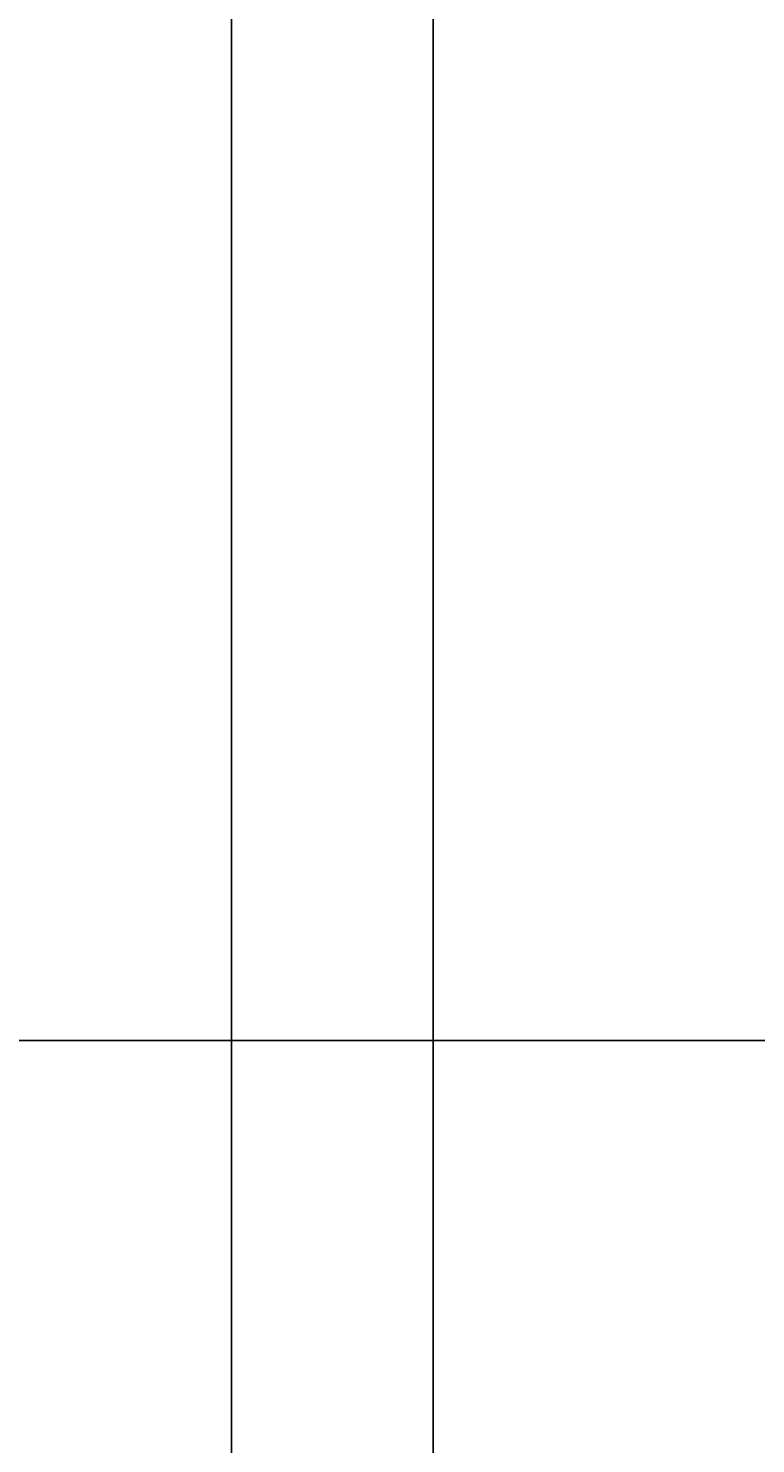
# Model space of a CAD drawing. Units: inches. Extents: x 37 to 706, y -568 to 110.
# Tile 13 of 24: x 494 to 526, y -468 to -405. Entities that reach past the tile are written whole.
import ezdxf

# ---------------------------------------------------------------- set-up
doc = ezdxf.new("R2010")
doc.units = ezdxf.units.IN
doc.header["$MEASUREMENT"] = 0
doc.layers.add('A-ANNO-DIMS', color=2, linetype='Continuous', lineweight=18)
doc.styles.get("Standard").update_dxf_attribs({"font": 'arial.ttf'})
doc.dimstyles.get("Standard").update_dxf_attribs({"dimtxt": 0.18, "dimasz": 0.18, "dimexe": 0.18, "dimexo": 0.0625, "dimgap": 0.09, "dimtad": 0, "dimtih": 1, "dimtoh": 1, "dimdec": 0, "dimzin": 0, "dimdsep": 46, "dimlunit": 3, "dimtxsty": 'Standard', "dimcen": 0.09, "dimadec": 0, "dimazin": 0, "dimtfac": 1, "dimtdec": 0, "dimtofl": 0, "dimtmove": 0, "dimatfit": 3, "dimfxl": 1, "dimtolj": 1, "dimtzin": 0, "dimarcsym": 0})

# ---------------------------------------------------------------- blocks, each defined once
blk = doc.blocks.new('*D45')
at = {"layer": 'A-ANNO-DIMS', "color": 0, "lineweight": -2, "transparency": 16777216}
for p, q in [((88.021, -449.708), (705.888, -449.708)), ((705.708, -449.888), (705.708, -481.527)), ((705.708, -513.528), (705.708, -481.89)), ((79.021, -513.708), (705.888, -513.708))]:
    blk.add_line(p, q, dxfattribs=at)
at = {"layer": 'A-ANNO-DIMS', "color": 0, "transparency": 16777216}
for points in [[(705.678, -449.888), (705.738, -449.888), (705.708, -449.708)], [(705.678, -513.528), (705.738, -513.528), (705.708, -513.708)]]:
    blk.add_solid(points, dxfattribs=at)
at = {"layer": 'Defpoints', "color": 0, "transparency": 16777216}
for p in [(87.958, -449.708), (705.708, -449.708), (78.958, -513.708)]:
    blk.add_point(p, dxfattribs=at)
at = {"layer": 'A-ANNO-DIMS', "color": 0, "transparency": 16777216, "insert": (705.708, -481.708), "char_height": 0.18, "attachment_point": 5}
blk.add_mtext('\\A1;5\'-4"', dxfattribs=at)
blk = doc.blocks.new('*D53')
at = {"layer": 'A-ANNO-DIMS', "color": 0, "lineweight": -2, "transparency": 16777216}
for p, q in [((511.958, -151.771), (511.958, -567.638)), ((537.958, -151.771), (537.958, -567.638)), ((512.138, -567.458), (524.628, -567.458)), ((537.778, -567.458), (525.289, -567.458))]:
    blk.add_line(p, q, dxfattribs=at)
at = {"layer": 'A-ANNO-DIMS', "color": 0, "transparency": 16777216}
for points in [[(512.138, -567.428), (512.138, -567.488), (511.958, -567.458)], [(537.778, -567.428), (537.778, -567.488), (537.958, -567.458)]]:
    blk.add_solid(points, dxfattribs=at)
at = {"layer": 'Defpoints', "color": 0, "transparency": 16777216}
for p in [(511.958, -151.708), (537.958, -151.708), (537.958, -567.458)]:
    blk.add_point(p, dxfattribs=at)
at = {"layer": 'A-ANNO-DIMS', "color": 0, "transparency": 16777216, "insert": (524.958, -567.458), "char_height": 0.18, "attachment_point": 5}
blk.add_mtext('\\A1;2\'-2"', dxfattribs=at)
blk = doc.blocks.new('*D63')
at = {"layer": 'A-ANNO-DIMS', "color": 0, "lineweight": -2, "transparency": 16777216}
for p, q in [((478.958, -142.771), (478.958, -567.638)), ((502.958, -151.771), (502.958, -567.638)), ((479.138, -567.458), (490.628, -567.458)), ((502.778, -567.458), (491.289, -567.458))]:
    blk.add_line(p, q, dxfattribs=at)
at = {"layer": 'A-ANNO-DIMS', "color": 0, "transparency": 16777216}
for points in [[(479.138, -567.428), (479.138, -567.488), (478.958, -567.458)], [(502.778, -567.428), (502.778, -567.488), (502.958, -567.458)]]:
    blk.add_solid(points, dxfattribs=at)
at = {"layer": 'Defpoints', "color": 0, "transparency": 16777216}
for p in [(478.958, -142.708), (502.958, -151.708), (502.958, -567.458)]:
    blk.add_point(p, dxfattribs=at)
at = {"layer": 'A-ANNO-DIMS', "color": 0, "transparency": 16777216, "insert": (490.958, -567.458), "char_height": 0.18, "attachment_point": 5}
blk.add_mtext('\\A1;2\'-0"', dxfattribs=at)

msp = doc.modelspace()

# ---------------------------------------------------------------- dimensions: what is measured, and where the dimension line sits
at = {"layer": 'A-ANNO-DIMS'}
for base, p1, p2, picture, middle in [((502.958, -567.458), (478.958, -142.708), (502.958, -151.708), '*D63', (490.958, -567.458)), ((537.958, -567.458), (511.958, -151.708), (537.958, -151.708), '*D53', (524.958, -567.458))]:
    dim = msp.add_linear_dim(base=base, p1=p1, p2=p2, dimstyle='Standard', override={"dimdec": 1, "dimlfac": 1, "dimrnd": 0, "dimzin": 1, "dimdsep": 46, "dimlunit": 4, "dimfrac": 2}, dxfattribs=at)
    dim.commit()
    dim.dimension.update_dxf_attribs({"geometry": picture, "text_midpoint": middle})
dim = msp.add_linear_dim(base=(705.708, -449.708), p1=(78.958, -513.708), p2=(87.958, -449.708), angle=90, dimstyle='Standard', override={"dimdec": 1, "dimlfac": 1, "dimrnd": 0, "dimzin": 1, "dimdsep": 46, "dimlunit": 4, "dimfrac": 2}, dxfattribs=at)
dim.commit()
dim.dimension.update_dxf_attribs({"geometry": '*D45', "text_midpoint": (705.708, -481.708)})

doc.saveas('drawing.dxf')
